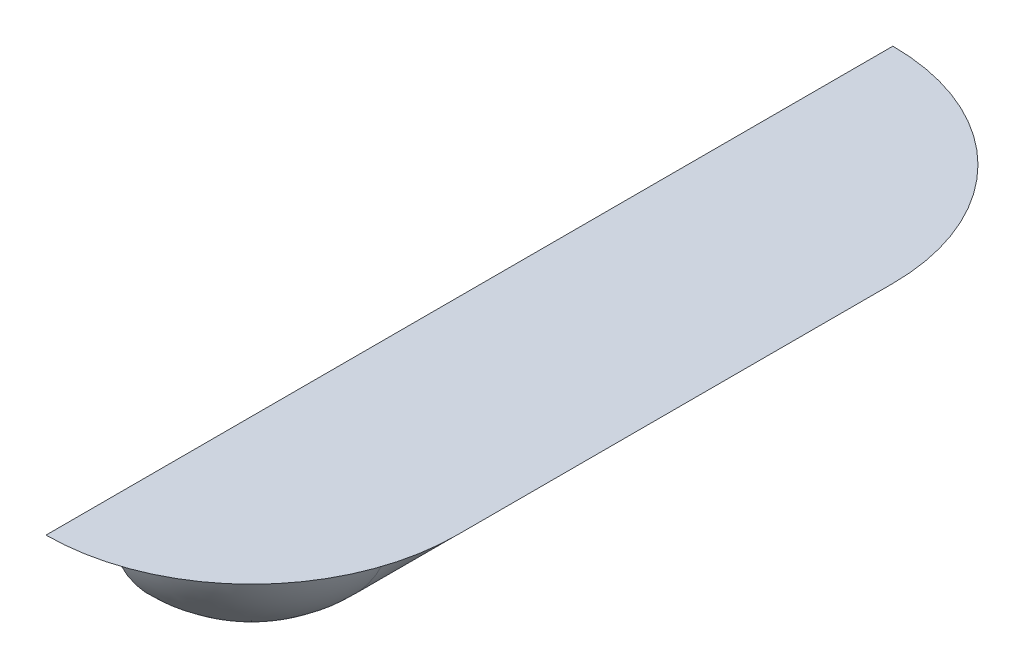
ISO-10303-21;
HEADER;
FILE_DESCRIPTION(('STEP AP214'),'2;1');
FILE_NAME('part.step','',(''),(''),'','','');
FILE_SCHEMA(('AUTOMOTIVE_DESIGN { 1 0 10303 214 1 1 1 1 }'));
ENDSEC;
DATA;
#1=APPLICATION_CONTEXT('core data for automotive mechanical design processes');
#2=APPLICATION_PROTOCOL_DEFINITION('international standard','automotive_design',2000,#1);
#3=PRODUCT_CONTEXT('',#1,'mechanical');
#4=PRODUCT('Part','Part','',(#3));
#5=PRODUCT_RELATED_PRODUCT_CATEGORY('part','',(#4));
#6=PRODUCT_DEFINITION_FORMATION('','',#4);
#7=PRODUCT_DEFINITION_CONTEXT('part definition',#1,'design');
#8=PRODUCT_DEFINITION('design','',#6,#7);
#9=PRODUCT_DEFINITION_SHAPE('','',#8);
#10=(LENGTH_UNIT() NAMED_UNIT(*) SI_UNIT(.MILLI.,.METRE.));
#11=(NAMED_UNIT(*) PLANE_ANGLE_UNIT() SI_UNIT($,.RADIAN.));
#12=(NAMED_UNIT(*) SI_UNIT($,.STERADIAN.) SOLID_ANGLE_UNIT());
#13=UNCERTAINTY_MEASURE_WITH_UNIT(LENGTH_MEASURE(1.E-05),#10,'distance_accuracy_value','');
#14=(GEOMETRIC_REPRESENTATION_CONTEXT(3) GLOBAL_UNCERTAINTY_ASSIGNED_CONTEXT((#13)) GLOBAL_UNIT_ASSIGNED_CONTEXT((#10,
#11,#12)) REPRESENTATION_CONTEXT('',''));
#15=CARTESIAN_POINT('',(0.,0.,0.));
#16=DIRECTION('',(0.,0.,1.));
#17=DIRECTION('',(1.,0.,0.));
#18=AXIS2_PLACEMENT_3D('',#15,#16,#17);
#19=CARTESIAN_POINT('',(-10.,0.,30.));
#20=DIRECTION('',(1.,0.,0.));
#21=DIRECTION('',(0.,1.,0.));
#22=AXIS2_PLACEMENT_3D('',#19,#20,#21);
#23=PLANE('',#22);
#24=DIRECTION('',(0.,0.,-1.));
#25=VECTOR('',#24,1.);
#26=CARTESIAN_POINT('',(-10.,0.,30.));
#27=LINE('',#26,#25);
#28=CARTESIAN_POINT('',(-10.,0.,58.2842712474619));
#29=VERTEX_POINT('',#28);
#30=CARTESIAN_POINT('',(-10.,0.,-58.2842712474619));
#31=VERTEX_POINT('',#30);
#32=EDGE_CURVE('E101',#29,#31,#27,.T.);
#33=ORIENTED_EDGE('',*,*,#32,.T.);
#34=CARTESIAN_POINT('',(-10.,-10.,-58.2842712474619));
#35=DIRECTION('',(1.,0.,0.));
#36=DIRECTION('',(0.,1.,0.));
#37=AXIS2_PLACEMENT_3D('',#34,#35,#36);
#38=CIRCLE('',#37,10.);
#39=CARTESIAN_POINT('',(-10.0000000000001,-6.66666666666667,-48.8561808316413));
#40=VERTEX_POINT('',#39);
#41=EDGE_CURVE('E11',#31,#40,#38,.T.);
#42=ORIENTED_EDGE('',*,*,#41,.T.);
#43=CARTESIAN_POINT('',(-10.,0.,-30.));
#44=DIRECTION('',(-1.,0.,0.));
#45=DIRECTION('',(0.,0.,1.));
#46=AXIS2_PLACEMENT_3D('',#43,#44,#45);
#47=CIRCLE('',#46,20.);
#48=CARTESIAN_POINT('',(-10.,-20.,-30.));
#49=VERTEX_POINT('',#48);
#50=EDGE_CURVE('E137',#40,#49,#47,.T.);
#51=ORIENTED_EDGE('',*,*,#50,.T.);
#52=DIRECTION('',(0.,0.,-1.));
#53=VECTOR('',#52,1.);
#54=CARTESIAN_POINT('',(-10.,-20.,30.));
#55=LINE('',#54,#53);
#56=CARTESIAN_POINT('',(-10.,-20.,30.));
#57=VERTEX_POINT('',#56);
#58=EDGE_CURVE('E135',#57,#49,#55,.T.);
#59=ORIENTED_EDGE('',*,*,#58,.F.);
#60=CARTESIAN_POINT('',(-10.,0.,30.));
#61=DIRECTION('',(-1.,0.,0.));
#62=DIRECTION('',(0.,0.,1.));
#63=AXIS2_PLACEMENT_3D('',#60,#61,#62);
#64=CIRCLE('',#63,20.);
#65=CARTESIAN_POINT('',(-10.0000000000001,-6.66666666666667,48.8561808316413));
#66=VERTEX_POINT('',#65);
#67=EDGE_CURVE('E129',#57,#66,#64,.T.);
#68=ORIENTED_EDGE('',*,*,#67,.T.);
#69=CARTESIAN_POINT('',(-10.,-10.,58.2842712474619));
#70=DIRECTION('',(1.,0.,0.));
#71=DIRECTION('',(0.,1.,0.));
#72=AXIS2_PLACEMENT_3D('',#69,#70,#71);
#73=CIRCLE('',#72,10.);
#74=EDGE_CURVE('E59',#66,#29,#73,.T.);
#75=ORIENTED_EDGE('',*,*,#74,.T.);
#76=EDGE_LOOP('',(#33,#42,#51,#59,#68,#75));
#77=FACE_BOUND('',#76,.T.);
#78=ADVANCED_FACE('F47',(#77),#23,.F.);
#79=CARTESIAN_POINT('',(-10.,0.,30.));
#80=DIRECTION('',(0.,0.,-1.));
#81=DIRECTION('',(-1.,0.,0.));
#82=AXIS2_PLACEMENT_3D('',#79,#80,#81);
#83=CYLINDRICAL_SURFACE('',#82,20.);
#84=CARTESIAN_POINT('',(-10.,0.,-30.));
#85=DIRECTION('',(0.,0.,1.));
#86=DIRECTION('',(1.,0.,0.));
#87=AXIS2_PLACEMENT_3D('',#84,#85,#86);
#88=CIRCLE('',#87,20.);
#89=CARTESIAN_POINT('',(8.85618083164128,-6.66666666666667,-30.));
#90=VERTEX_POINT('',#89);
#91=EDGE_CURVE('E134',#49,#90,#88,.T.);
#92=ORIENTED_EDGE('',*,*,#91,.T.);
#93=DIRECTION('',(0.,0.,-1.));
#94=VECTOR('',#93,1.);
#95=CARTESIAN_POINT('',(8.85618083164128,-6.66666666666667,30.));
#96=LINE('',#95,#94);
#97=CARTESIAN_POINT('',(8.85618083164128,-6.66666666666667,30.));
#98=VERTEX_POINT('',#97);
#99=EDGE_CURVE('E121',#90,#98,#96,.F.);
#100=ORIENTED_EDGE('',*,*,#99,.T.);
#101=CARTESIAN_POINT('',(-10.,0.,30.));
#102=DIRECTION('',(0.,0.,1.));
#103=DIRECTION('',(1.,0.,0.));
#104=AXIS2_PLACEMENT_3D('',#101,#102,#103);
#105=CIRCLE('',#104,20.);
#106=EDGE_CURVE('E140',#57,#98,#105,.T.);
#107=ORIENTED_EDGE('',*,*,#106,.F.);
#108=ORIENTED_EDGE('',*,*,#58,.T.);
#109=EDGE_LOOP('',(#92,#100,#107,#108));
#110=FACE_BOUND('',#109,.T.);
#111=ADVANCED_FACE('F144',(#110),#83,.T.);
#112=CARTESIAN_POINT('',(-10.,0.,30.));
#113=DIRECTION('',(0.,1.,0.));
#114=DIRECTION('',(0.,0.,-1.));
#115=AXIS2_PLACEMENT_3D('',#112,#113,#114);
#116=SPHERICAL_SURFACE('',#115,20.);
#117=ORIENTED_EDGE('',*,*,#106,.T.);
#118=CARTESIAN_POINT('',(-10.,-6.66666666666667,30.));
#119=DIRECTION('',(0.,1.,0.));
#120=DIRECTION('',(0.,0.,1.));
#121=AXIS2_PLACEMENT_3D('',#118,#119,#120);
#122=CIRCLE('',#121,18.8561808316413);
#123=EDGE_CURVE('E110',#98,#66,#122,.F.);
#124=ORIENTED_EDGE('',*,*,#123,.T.);
#125=ORIENTED_EDGE('',*,*,#67,.F.);
#126=EDGE_LOOP('',(#117,#124,#125));
#127=FACE_BOUND('',#126,.T.);
#128=ADVANCED_FACE('F143',(#127),#116,.T.);
#129=CARTESIAN_POINT('',(-10.,0.,-30.));
#130=DIRECTION('',(0.,-1.,0.));
#131=DIRECTION('',(0.,0.,-1.));
#132=AXIS2_PLACEMENT_3D('',#129,#130,#131);
#133=SPHERICAL_SURFACE('',#132,20.);
#134=ORIENTED_EDGE('',*,*,#50,.F.);
#135=CARTESIAN_POINT('',(-10.,-6.66666666666667,-30.));
#136=DIRECTION('',(0.,1.,0.));
#137=DIRECTION('',(0.,0.,1.));
#138=AXIS2_PLACEMENT_3D('',#135,#136,#137);
#139=CIRCLE('',#138,18.8561808316413);
#140=EDGE_CURVE('E72',#40,#90,#139,.F.);
#141=ORIENTED_EDGE('',*,*,#140,.T.);
#142=ORIENTED_EDGE('',*,*,#91,.F.);
#143=EDGE_LOOP('',(#134,#141,#142));
#144=FACE_BOUND('',#143,.T.);
#145=ADVANCED_FACE('F150',(#144),#133,.T.);
#146=CARTESIAN_POINT('',(-10.,-10.,-30.));
#147=DIRECTION('',(0.,1.,0.));
#148=DIRECTION('',(0.,0.,1.));
#149=AXIS2_PLACEMENT_3D('',#146,#147,#148);
#150=TOROIDAL_SURFACE('',#149,28.2842712474619,10.);
#151=ORIENTED_EDGE('',*,*,#41,.F.);
#152=CARTESIAN_POINT('',(-10.,0.,-30.));
#153=DIRECTION('',(0.,1.,0.));
#154=DIRECTION('',(0.,0.,1.));
#155=AXIS2_PLACEMENT_3D('',#152,#153,#154);
#156=CIRCLE('',#155,28.2842712474619);
#157=CARTESIAN_POINT('',(18.2842712474619,0.,-30.));
#158=VERTEX_POINT('',#157);
#159=EDGE_CURVE('E117',#158,#31,#156,.T.);
#160=ORIENTED_EDGE('',*,*,#159,.F.);
#161=CARTESIAN_POINT('',(18.2842712474619,-10.,-30.));
#162=DIRECTION('',(0.,0.,-1.));
#163=DIRECTION('',(0.,1.,0.));
#164=AXIS2_PLACEMENT_3D('',#161,#162,#163);
#165=CIRCLE('',#164,10.);
#166=EDGE_CURVE('E52',#90,#158,#165,.T.);
#167=ORIENTED_EDGE('',*,*,#166,.F.);
#168=ORIENTED_EDGE('',*,*,#140,.F.);
#169=EDGE_LOOP('',(#151,#160,#167,#168));
#170=FACE_BOUND('',#169,.T.);
#171=ADVANCED_FACE('F51',(#170),#150,.F.);
#172=CARTESIAN_POINT('',(18.2842712474619,-10.,30.));
#173=DIRECTION('',(0.,0.,-1.));
#174=DIRECTION('',(-1.,0.,0.));
#175=AXIS2_PLACEMENT_3D('',#172,#173,#174);
#176=CYLINDRICAL_SURFACE('',#175,10.);
#177=ORIENTED_EDGE('',*,*,#166,.T.);
#178=DIRECTION('',(0.,0.,1.));
#179=VECTOR('',#178,1.);
#180=CARTESIAN_POINT('',(18.2842712474619,0.,-30.));
#181=LINE('',#180,#179);
#182=CARTESIAN_POINT('',(18.2842712474619,0.,30.));
#183=VERTEX_POINT('',#182);
#184=EDGE_CURVE('E103',#183,#158,#181,.F.);
#185=ORIENTED_EDGE('',*,*,#184,.F.);
#186=CARTESIAN_POINT('',(18.2842712474619,-10.,30.));
#187=DIRECTION('',(0.,0.,-1.));
#188=DIRECTION('',(0.,1.,0.));
#189=AXIS2_PLACEMENT_3D('',#186,#187,#188);
#190=CIRCLE('',#189,10.);
#191=EDGE_CURVE('E111',#98,#183,#190,.T.);
#192=ORIENTED_EDGE('',*,*,#191,.F.);
#193=ORIENTED_EDGE('',*,*,#99,.F.);
#194=EDGE_LOOP('',(#177,#185,#192,#193));
#195=FACE_BOUND('',#194,.T.);
#196=ADVANCED_FACE('F116',(#195),#176,.F.);
#197=CARTESIAN_POINT('',(-10.,-10.,30.));
#198=DIRECTION('',(0.,1.,0.));
#199=DIRECTION('',(0.,0.,1.));
#200=AXIS2_PLACEMENT_3D('',#197,#198,#199);
#201=TOROIDAL_SURFACE('',#200,28.2842712474619,10.);
#202=ORIENTED_EDGE('',*,*,#74,.F.);
#203=ORIENTED_EDGE('',*,*,#123,.F.);
#204=ORIENTED_EDGE('',*,*,#191,.T.);
#205=CARTESIAN_POINT('',(-10.,0.,30.));
#206=DIRECTION('',(0.,1.,0.));
#207=DIRECTION('',(0.,0.,1.));
#208=AXIS2_PLACEMENT_3D('',#205,#206,#207);
#209=CIRCLE('',#208,28.2842712474619);
#210=EDGE_CURVE('E97',#29,#183,#209,.T.);
#211=ORIENTED_EDGE('',*,*,#210,.F.);
#212=EDGE_LOOP('',(#202,#203,#204,#211));
#213=FACE_BOUND('',#212,.T.);
#214=ADVANCED_FACE('F115',(#213),#201,.F.);
#215=CARTESIAN_POINT('',(25.,0.,-75.));
#216=DIRECTION('',(0.,-1.,0.));
#217=DIRECTION('',(0.,0.,-1.));
#218=AXIS2_PLACEMENT_3D('',#215,#216,#217);
#219=PLANE('',#218);
#220=ORIENTED_EDGE('',*,*,#210,.T.);
#221=ORIENTED_EDGE('',*,*,#184,.T.);
#222=ORIENTED_EDGE('',*,*,#159,.T.);
#223=ORIENTED_EDGE('',*,*,#32,.F.);
#224=EDGE_LOOP('',(#220,#221,#222,#223));
#225=FACE_BOUND('',#224,.T.);
#226=ADVANCED_FACE('F100',(#225),#219,.F.);
#227=CLOSED_SHELL('',(#78,#111,#128,#145,#171,#196,#214,#226));
#228=MANIFOLD_SOLID_BREP('B2',#227);
#229=ADVANCED_BREP_SHAPE_REPRESENTATION('',(#18,#228),#14);
#230=SHAPE_DEFINITION_REPRESENTATION(#9,#229);
ENDSEC;
END-ISO-10303-21;
